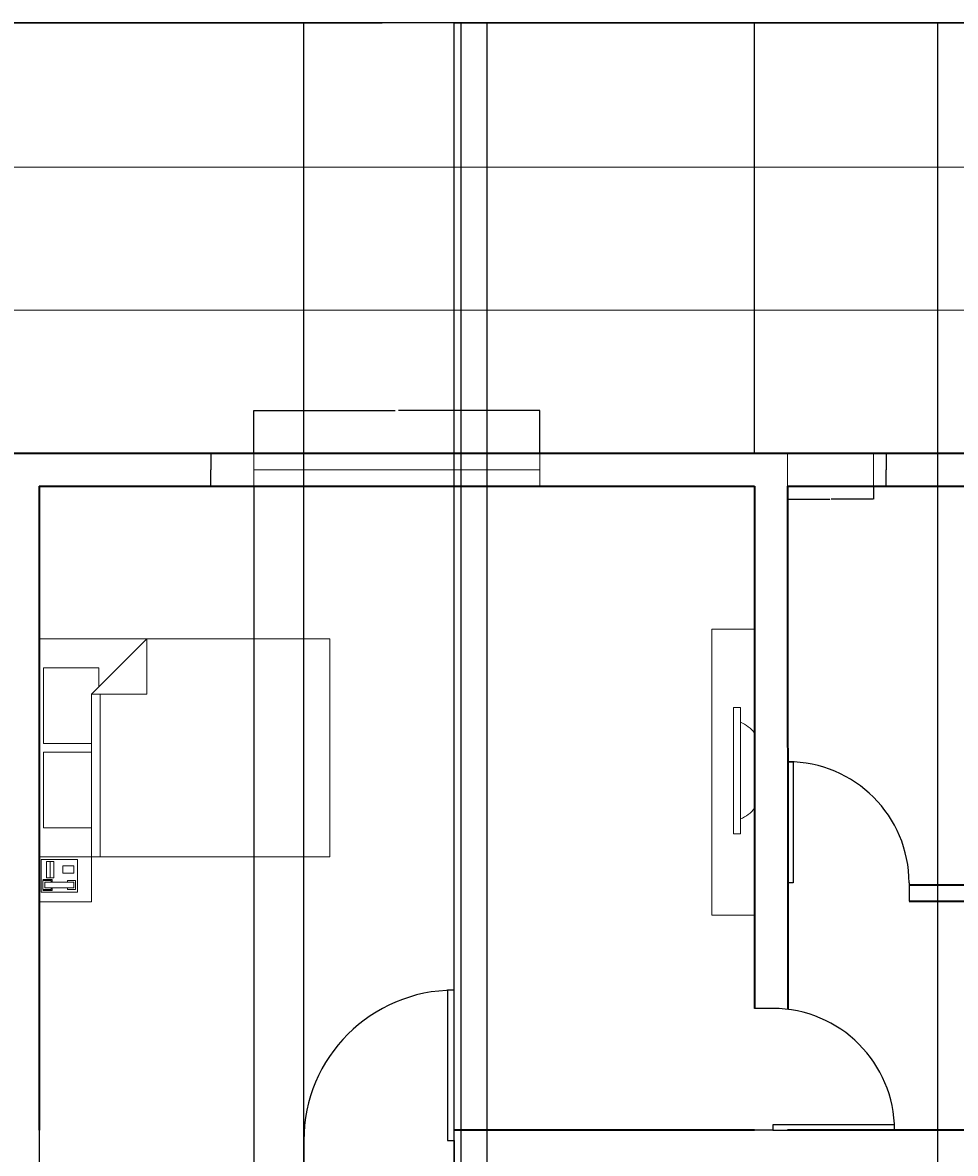
# Model space of a CAD drawing. Units: millimetres. Extents: x -8052 to 19968, y -37825 to -17505.
# Tile 8 of 10: x 4015 to 10533, y -25407 to -17505. Entities that reach past the tile are written whole.
import ezdxf

# ---------------------------------------------------------------- set-up
doc = ezdxf.new("R2010")
doc.units = ezdxf.units.MM
doc.header["$MEASUREMENT"] = 0
for name, color, linetype, lineweight in [('A-ANNO-DIMS', 2, 'Continuous', 18), ('A-DOOR', 3, 'Continuous', 25), ('A-EQPM', 8, 'Continuous', 18), ('A-FLOR', 8, 'Continuous', 18), ('A-FURN', 8, 'Continuous', 18), ('A-GLAZ', 4, 'Continuous', 18), ('A-WALL', 7, 'Continuous', 35)]:
    doc.layers.add(name, color=color, linetype=linetype, lineweight=lineweight)
doc.styles.get("Standard").update_dxf_attribs({"font": 'arial.ttf'})
doc.dimstyles.get("Standard").update_dxf_attribs({"dimtxt": 1.054, "dimasz": 1.055, "dimexe": 0.18, "dimexo": 0.0625, "dimgap": 0.09, "dimtad": 0, "dimtih": 1, "dimtoh": 1, "dimdec": 4, "dimzin": 0, "dimdsep": 46, "dimtxsty": 'Standard', "dimcen": 0.09, "dimadec": 0, "dimazin": 0, "dimtfac": 1, "dimtdec": 4, "dimtofl": 0, "dimtmove": 0, "dimatfit": 3, "dimfxl": 1, "dimtolj": 1, "dimtzin": 0, "dimarcsym": 0})

# ---------------------------------------------------------------- blocks, each defined once
blk = doc.blocks.new('*U9')
for p, q in [((-40, 0), (-40, 6)), ((0, 0), (0, 6))]:
    blk.add_line(p, q)
blk.add_lwpolyline([(0, 0), (0, -40), (-1.75, -40), (-1.75, 0)], close=True)
blk.add_arc((0, 0), 40, 180, 270)
blk = doc.blocks.new('Bed - Queen')
for p, q in [((0, -80.00003), (0, 0)), ((0, 0), (59.99999, 0)), ((59.99999, 0), (59.99999, -80.00003)), ((7.99999, -1.2), (28.79998, -1.2)), ((7.99999, -14.4), (7.99999, -1.2)), ((28.79998, -1.2), (28.79998, -14.4)), ((31.19999, -1.2), (51.99999, -1.2)), ((31.19999, -14.4), (31.19999, -1.2)), ((51.99999, -1.2), (51.99999, -16.4)), ((0, -14.4), (44.8, -14.4)), ((59.99999, -29.6), (44.8, -14.4)), ((44.8, -14.4), (44.8, -29.6)), ((44.8, -16.8), (0, -16.8)), ((51.99999, -16.4), (46.79936, -16.4)), ((44.8, -29.6), (59.99999, -29.6)), ((59.99999, -80.00003), (0, -80.00003))]:
    blk.add_line(p, q)
blk = doc.blocks.new('Phone - Desk')
for p, q in [((-4.5, -5), (-4.5, 5)), ((-4.5, 5), (4.5, 5)), ((-4, 4.5), (-4, 2)), ((-3.75, 4.5), (-3.75, 2.25)), ((-1.25, 4.5), (-3.75, 4.5)), ((-3.25, 4), (-3.25, -4)), ((-3.25, 4), (-1.75, 4)), ((-1.75, -4), (-1.75, 4)), ((-1.25, 2.25), (-1.25, 4.5)), ((-1, 2), (-1, 4.5)), ((4, 3.5), (-0.5, 3.5)), ((-0.5, 3.5), (-0.5, 1.5)), ((4, 1.5), (4, 3.5)), ((4.5, 5), (4.5, -5)), ((-4, 2), (-3.25, 2)), ((-3.75, 2.25), (-3.25, 2.25)), ((-1.75, 2.25), (-1.25, 2.25)), ((-1.75, 2), (-1, 2)), ((-0.5, 2.5), (4, 2.5)), ((-0.5, 1.5), (4, 1.5)), ((-3.75, -2.25), (-3.25, -2.25)), ((-3.75, -4.5), (-3.75, -2.25)), ((-1.75, -2.25), (-1.25, -2.25)), ((-1.25, -2.25), (-1.25, -4.5)), ((2.75, -1), (0.75, -1)), ((0.75, -1), (0.75, -4)), ((2.75, -4), (2.75, -1)), ((4.5, -5), (-4.5, -5)), ((-1.25, -4.5), (-3.75, -4.5)), ((-3.25, -4), (-1.75, -4)), ((0.75, -4), (2.75, -4))]:
    blk.add_line(p, q)
blk = doc.blocks.new('*U20')
for p, q in [((0, 0), (0, -6)), ((-40, 0), (-40, -6))]:
    blk.add_line(p, q)
blk.add_lwpolyline([(0, 0), (0, 40), (-1.75, 40), (-1.75, 0)], close=True)
blk.add_arc((0, 0), 40, 90, 180)
blk = doc.blocks.new('TABLE-BEDSIDE')
for p, q in [((365.8, 315.3), (365.8, 0)), ((365.8, 0), (0, 0))]:
    blk.add_line(p, q)
blk = doc.blocks.new('MEDIA-CONSOLE-2000')
for points in [[(300, 2000), (0, 2000), (0, 0), (300, 0)], [(201.6, 1452.1), (152.5, 1452.1), (152.5, 569.2), (201.6, 569.2)], [(201.6, 569.2), (152.5, 569.2), (152.5, 1452.1), (201.6, 1452.1)]]:
    blk.add_lwpolyline(points, close=True)
for centre, start, end in [((115.1, 1133.4), 37.07446, 68.10078), ((115.1, 887.8), 291.89922, 322.92554)]:
    blk.add_arc(centre, 231.7, start, end)
blk = doc.blocks.new('DOOR-SWING-850')
for p, q in [((0, 127.5), (0, 0)), ((850, 127.5), (850, 0))]:
    blk.add_line(p, q)
blk.add_lwpolyline([(850, 127.5), (850, 977.5), (812.8, 977.5), (812.8, 127.5)], close=True)
blk.add_arc((850, 127.5), 850, 90, 180)
blk = doc.blocks.new('WIN-2000')
for p, q in [((0, 0), (0, 230)), ((2000, 0), (2000, 230)), ((0, 115), (2000, 115))]:
    blk.add_line(p, q)
blk = doc.blocks.new('VENT-OPENING-600')
for p, q in [((0, 0), (0, 230)), ((600, 0), (600, 230))]:
    blk.add_line(p, q)
blk = doc.blocks.new('*D52')
at = {"layer": 'A-ANNO-DIMS', "color": 0, "lineweight": -2, "transparency": 16777216}
for p, q in [((5630, -20514.8), (5630, -20214.7)), ((5631, -20214.8), (6619.1, -20214.8)), ((7628.9, -20214.8), (6640.9, -20214.8)), ((7630, -20514.8), (7630, -20214.7))]:
    blk.add_line(p, q, dxfattribs=at)
at = {"layer": 'A-ANNO-DIMS', "color": 0, "lineweight": 100, "transparency": 16777216}
for points in [[(5631, -20214.7), (5631, -20215), (5630, -20214.8)], [(7628.9, -20214.7), (7628.9, -20215), (7630, -20214.8)]]:
    blk.add_solid(points, dxfattribs=at)
at = {"layer": 'Defpoints', "color": 0, "lineweight": 100, "transparency": 16777216}
for p in [(5630, -20214.8), (5630, -20514.8), (7630, -20514.8)]:
    blk.add_point(p, dxfattribs=at)
at = {"layer": 'A-ANNO-DIMS', "color": 0, "transparency": 16777216, "insert": (6630, -20214.8), "char_height": 1.054, "attachment_point": 5}
blk.add_mtext('\\A1;BEDROOM WINDOW 2000 TYP.', dxfattribs=at)
blk = doc.blocks.new('*D53')
at = {"layer": 'A-ANNO-DIMS', "color": 0, "lineweight": -2, "transparency": 16777216}
for p, q in [((5629.9, -20514.8), (5329.8, -20514.8)), ((5330, -20515.9), (5330, -20629.2)), ((5330, -20743.8), (5330, -20630.5)), ((5629.9, -20744.8), (5329.8, -20744.8))]:
    blk.add_line(p, q, dxfattribs=at)
at = {"layer": 'A-ANNO-DIMS', "color": 0, "lineweight": 100, "transparency": 16777216}
for points in [[(5329.8, -20515.9), (5330.2, -20515.9), (5330, -20514.8)], [(5329.8, -20743.8), (5330.2, -20743.8), (5330, -20744.8)]]:
    blk.add_solid(points, dxfattribs=at)
at = {"layer": 'Defpoints', "color": 0, "lineweight": 100, "transparency": 16777216}
for p in [(5630, -20514.8), (5330, -20744.8), (5630, -20744.8)]:
    blk.add_point(p, dxfattribs=at)
at = {"layer": 'A-ANNO-DIMS', "color": 0, "transparency": 16777216, "insert": (5330, -20629.8), "char_height": 1.054, "attachment_point": 5}
blk.add_mtext('\\A1;230 TYP.', dxfattribs=at)
blk = doc.blocks.new('*D64')
at = {"layer": 'A-ANNO-DIMS', "color": 0, "lineweight": -2, "transparency": 16777216}
for p, q in [((9360, -20744.9), (9360, -20835)), ((9960, -20744.9), (9960, -20835)), ((9361, -20834.8), (9654.7, -20834.8)), ((9958.9, -20834.8), (9665.2, -20834.8))]:
    blk.add_line(p, q, dxfattribs=at)
at = {"layer": 'A-ANNO-DIMS', "color": 0, "lineweight": 100, "transparency": 16777216}
for points in [[(9361, -20834.7), (9361, -20835), (9360, -20834.8)], [(9958.9, -20834.7), (9958.9, -20835), (9960, -20834.8)]]:
    blk.add_solid(points, dxfattribs=at)
at = {"layer": 'Defpoints', "color": 0, "lineweight": 100, "transparency": 16777216}
for p in [(9360, -20744.8), (9960, -20744.8), (9960, -20834.8)]:
    blk.add_point(p, dxfattribs=at)
at = {"layer": 'A-ANNO-DIMS', "color": 0, "transparency": 16777216, "insert": (9660, -20834.8), "char_height": 1.054, "attachment_point": 5}
blk.add_mtext('\\A1;VENT 600 TYP.', dxfattribs=at)
blk = doc.blocks.new('*D65')
at = {"layer": 'A-ANNO-DIMS', "color": 0, "lineweight": -2, "transparency": 16777216}
for p, q in [((9960, -20514.8), (10050.2, -20514.8)), ((10050, -20515.9), (10050, -20629.2)), ((10050, -20743.8), (10050, -20630.5)), ((9960, -20744.8), (10050.2, -20744.8))]:
    blk.add_line(p, q, dxfattribs=at)
at = {"layer": 'A-ANNO-DIMS', "color": 0, "lineweight": 100, "transparency": 16777216}
for points in [[(10049.8, -20515.9), (10050.2, -20515.9), (10050, -20514.8)], [(10049.8, -20743.8), (10050.2, -20743.8), (10050, -20744.8)]]:
    blk.add_solid(points, dxfattribs=at)
at = {"layer": 'Defpoints', "color": 0, "lineweight": 100, "transparency": 16777216}
for p in [(9960, -20514.8), (10050, -20514.8), (9960, -20744.8)]:
    blk.add_point(p, dxfattribs=at)
at = {"layer": 'A-ANNO-DIMS', "color": 0, "transparency": 16777216, "insert": (10050, -20629.8), "char_height": 1.054, "attachment_point": 5}
blk.add_mtext('\\A1;230 TYP.', dxfattribs=at)
blk = doc.blocks.new('*D84')
at = {"layer": 'A-ANNO-DIMS', "color": 0, "lineweight": -2, "transparency": 16777216}
for p, q in [((-7040, -18514.8), (-7040, -17505.2)), ((-7039, -17505.3), (3022.9, -17505.3)), ((13088.9, -17505.3), (3027.1, -17505.3)), ((13090, -18514.8), (13090, -17505.2))]:
    blk.add_line(p, q, dxfattribs=at)
at = {"layer": 'A-ANNO-DIMS', "color": 0, "lineweight": 100, "transparency": 16777216}
for points in [[(-7039, -17505.2), (-7039, -17505.5), (-7040, -17505.3)], [(13088.9, -17505.2), (13088.9, -17505.5), (13090, -17505.3)]]:
    blk.add_solid(points, dxfattribs=at)
at = {"layer": 'Defpoints', "color": 0, "lineweight": 100, "transparency": 16777216}
for p in [(13090, -17505.3), (-7040, -18514.8), (13090, -18514.8)]:
    blk.add_point(p, dxfattribs=at)
at = {"layer": 'A-ANNO-DIMS', "color": 0, "transparency": 16777216, "insert": (3025, -17505.3), "char_height": 1.05, "attachment_point": 5}
blk.add_mtext('\\A1;20130', dxfattribs=at)
blk = doc.blocks.new('*D92')
at = {"layer": 'A-ANNO-DIMS', "color": 0, "lineweight": -2, "transparency": 16777216}
for p, q in [((3900, -20514.8), (3900, -17505.2)), ((3901, -17505.3), (6513.3, -17505.3)), ((9128.9, -17505.3), (6516.6, -17505.3)), ((9130, -20514.8), (9130, -17505.2))]:
    blk.add_line(p, q, dxfattribs=at)
at = {"layer": 'A-ANNO-DIMS', "color": 0, "lineweight": 100, "transparency": 16777216}
for points in [[(3901, -17505.2), (3901, -17505.5), (3900, -17505.3)], [(9128.9, -17505.2), (9128.9, -17505.5), (9130, -17505.3)]]:
    blk.add_solid(points, dxfattribs=at)
at = {"layer": 'Defpoints', "color": 0, "lineweight": 100, "transparency": 16777216}
for p in [(9130, -17505.3), (3900, -20514.8), (9130, -20514.8)]:
    blk.add_point(p, dxfattribs=at)
at = {"layer": 'A-ANNO-DIMS', "color": 0, "transparency": 16777216, "insert": (6515, -17505.3), "char_height": 1.05, "attachment_point": 5}
blk.add_mtext('\\A1;5230', dxfattribs=at)
blk = doc.blocks.new('*D93')
at = {"layer": 'A-ANNO-DIMS', "color": 0, "lineweight": -2, "transparency": 16777216}
for p, q in [((9130, -20514.8), (9130, -17505.2)), ((9131, -17505.3), (10608.3, -17505.3)), ((12088.9, -17505.3), (10611.7, -17505.3)), ((12090, -20514.8), (12090, -17505.2))]:
    blk.add_line(p, q, dxfattribs=at)
at = {"layer": 'A-ANNO-DIMS', "color": 0, "lineweight": 100, "transparency": 16777216}
for points in [[(9131, -17505.2), (9131, -17505.5), (9130, -17505.3)], [(12088.9, -17505.2), (12088.9, -17505.5), (12090, -17505.3)]]:
    blk.add_solid(points, dxfattribs=at)
at = {"layer": 'Defpoints', "color": 0, "lineweight": 100, "transparency": 16777216}
for p in [(12090, -17505.3), (9130, -20514.8), (12090, -20514.8)]:
    blk.add_point(p, dxfattribs=at)
at = {"layer": 'A-ANNO-DIMS', "color": 0, "transparency": 16777216, "insert": (10610, -17505.3), "char_height": 1.05, "attachment_point": 5}
blk.add_mtext('\\A1;2960', dxfattribs=at)
blk = doc.blocks.new('*D95')
at = {"layer": 'A-ANNO-DIMS', "color": 0, "lineweight": -2, "transparency": 16777216}
for p, q in [((4130, -20744.9), (4130, -37824.5)), ((5630, -20744.9), (5630, -37824.5)), ((4131, -37824.3), (4878.4, -37824.3)), ((5628.9, -37824.3), (4881.6, -37824.3))]:
    blk.add_line(p, q, dxfattribs=at)
at = {"layer": 'A-ANNO-DIMS', "color": 0, "lineweight": 100, "transparency": 16777216}
for points in [[(4131, -37824.2), (4131, -37824.5), (4130, -37824.3)], [(5628.9, -37824.2), (5628.9, -37824.5), (5630, -37824.3)]]:
    blk.add_solid(points, dxfattribs=at)
at = {"layer": 'Defpoints', "color": 0, "lineweight": 100, "transparency": 16777216}
for p in [(4130, -20744.8), (5630, -20744.8), (5630, -37824.3)]:
    blk.add_point(p, dxfattribs=at)
at = {"layer": 'A-ANNO-DIMS', "color": 0, "transparency": 16777216, "insert": (4880, -37824.3), "char_height": 1.05, "attachment_point": 5}
blk.add_mtext('\\A1;1500', dxfattribs=at)
blk = doc.blocks.new('*D104')
at = {"layer": 'A-ANNO-DIMS', "color": 0, "lineweight": -2, "transparency": 16777216}
for p, q in [((5980, -35400), (5980, -17505.2)), ((5981, -17505.3), (6528.4, -17505.3)), ((7078.9, -17505.3), (6531.6, -17505.3)), ((7080, -35584.8), (7080, -17505.2))]:
    blk.add_line(p, q, dxfattribs=at)
at = {"layer": 'A-ANNO-DIMS', "color": 0, "lineweight": 100, "transparency": 16777216}
for points in [[(5981, -17505.2), (5981, -17505.5), (5980, -17505.3)], [(7078.9, -17505.2), (7078.9, -17505.5), (7080, -17505.3)]]:
    blk.add_solid(points, dxfattribs=at)
at = {"layer": 'Defpoints', "color": 0, "lineweight": 100, "transparency": 16777216}
for p in [(7080, -17505.3), (5980, -35400), (7080, -35584.8)]:
    blk.add_point(p, dxfattribs=at)
at = {"layer": 'A-ANNO-DIMS', "color": 0, "transparency": 16777216, "insert": (6530, -17505.3), "char_height": 1.05, "attachment_point": 5}
blk.add_mtext('\\A1;1100', dxfattribs=at)
blk = doc.blocks.new('*D108')
at = {"layer": 'A-ANNO-DIMS', "color": 0, "lineweight": -2, "transparency": 16777216}
for p, q in [((-330, -29974.8), (-330, -17505.2)), ((-329, -17505.3), (3348.3, -17505.3)), ((7028.9, -17505.3), (3351.6, -17505.3)), ((7030, -29974.8), (7030, -17505.2))]:
    blk.add_line(p, q, dxfattribs=at)
at = {"layer": 'A-ANNO-DIMS', "color": 0, "lineweight": 100, "transparency": 16777216}
for points in [[(-329, -17505.2), (-329, -17505.5), (-330, -17505.3)], [(7028.9, -17505.2), (7028.9, -17505.5), (7030, -17505.3)]]:
    blk.add_solid(points, dxfattribs=at)
at = {"layer": 'Defpoints', "color": 0, "lineweight": 100, "transparency": 16777216}
for p in [(7030, -17505.3), (-330, -29974.8), (7030, -29974.8)]:
    blk.add_point(p, dxfattribs=at)
at = {"layer": 'A-ANNO-DIMS', "color": 0, "transparency": 16777216, "insert": (3350, -17505.3), "char_height": 1.05, "attachment_point": 5}
blk.add_mtext('\\A1;7360', dxfattribs=at)
blk = doc.blocks.new('*D123')
at = {"layer": 'A-ANNO-DIMS', "color": 0, "lineweight": -2, "transparency": 16777216}
for p, q in [((7260, -25474.8), (7260, -17505.2)), ((7261, -17505.3), (9673.3, -17505.3)), ((12088.9, -17505.3), (9676.7, -17505.3)), ((12090, -25474.8), (12090, -17505.2))]:
    blk.add_line(p, q, dxfattribs=at)
at = {"layer": 'A-ANNO-DIMS', "color": 0, "lineweight": 100, "transparency": 16777216}
for points in [[(7261, -17505.2), (7261, -17505.5), (7260, -17505.3)], [(12088.9, -17505.2), (12088.9, -17505.5), (12090, -17505.3)]]:
    blk.add_solid(points, dxfattribs=at)
at = {"layer": 'Defpoints', "color": 0, "lineweight": 100, "transparency": 16777216}
for p in [(7260, -17505.3), (7260, -25474.8), (12090, -25474.8)]:
    blk.add_point(p, dxfattribs=at)
at = {"layer": 'A-ANNO-DIMS', "color": 0, "transparency": 16777216, "insert": (9675, -17505.3), "char_height": 1.05, "attachment_point": 5}
blk.add_mtext('\\A1;4830', dxfattribs=at)
blk = doc.blocks.new('*D124')
at = {"layer": 'A-ANNO-DIMS', "color": 0, "lineweight": -2, "transparency": 16777216}
for p, q in [((7030, -29974.8), (7030, -17505.2)), ((7031, -17505.3), (8718.3, -17505.3)), ((10408.9, -17505.3), (8721.6, -17505.3)), ((10410, -29974.8), (10410, -17505.2))]:
    blk.add_line(p, q, dxfattribs=at)
at = {"layer": 'A-ANNO-DIMS', "color": 0, "lineweight": 100, "transparency": 16777216}
for points in [[(7031, -17505.2), (7031, -17505.5), (7030, -17505.3)], [(10408.9, -17505.2), (10408.9, -17505.5), (10410, -17505.3)]]:
    blk.add_solid(points, dxfattribs=at)
at = {"layer": 'Defpoints', "color": 0, "lineweight": 100, "transparency": 16777216}
for p in [(10410, -17505.3), (7030, -29974.8), (10410, -29974.8)]:
    blk.add_point(p, dxfattribs=at)
at = {"layer": 'A-ANNO-DIMS', "color": 0, "transparency": 16777216, "insert": (8720, -17505.3), "char_height": 1.05, "attachment_point": 5}
blk.add_mtext('\\A1;3380', dxfattribs=at)

msp = doc.modelspace()

# ---------------------------------------------------------------- linework, layer by layer
at = {"layer": 'A-DOOR'}
msp.add_line((9359.979, -23517.343), (9359.979, -23644.843), dxfattribs=at)
at = {"layer": 'A-FLOR'}
for p, q in [((-4810.021, -18514.843), (13089.979, -18514.843)), ((-6040.021, -19514.843), (12089.979, -19514.843))]:
    msp.add_line(p, q, dxfattribs=at)
at = {"layer": 'A-WALL'}
for p, q in [((3899.979, -20514.843), (4129.979, -20514.843)), ((4129.979, -20514.843), (9129.979, -20514.843)), ((9129.979, -20514.843), (9359.979, -20514.843)), ((9359.979, -20514.843), (11859.979, -20514.843)), ((4129.979, -20744.843), (9129.979, -20744.843)), ((4129.979, -20744.843), (4129.979, -25244.843)), ((9129.979, -20744.843), (9129.979, -24394.843)), ((9359.979, -20744.843), (11859.979, -20744.843)), ((9359.979, -20744.843), (9361.771, -24401.265)), ((9359.979, -23529.843), (9361.401, -23529.843)), ((10209.02, -23529.843), (11859.979, -23529.843)), ((9359.979, -23644.843), (9361.401, -23644.843)), ((10209.02, -23644.843), (11859.979, -23644.843)), ((9129.979, -25244.843), (7029.979, -25244.843)), ((11859.979, -25244.843), (9359.979, -25244.843))]:
    msp.add_line(p, q, dxfattribs=at)

# ---------------------------------------------------------------- block references
at = {"layer": 'A-DOOR', "xscale": 21.1904853351297, "yscale": 21.1904853351297, "zscale": 21.1904853351297, "rotation": 180}
msp.add_blockref('*U9', (9361.401, -23517.7), dxfattribs=at)
at = {"layer": 'A-DOOR', "xscale": 26.25, "yscale": 26.25, "zscale": 26.25}
msp.add_blockref('*U20', (7029.979, -25317.343), dxfattribs=at)
at = {"layer": 'A-DOOR', "rotation": 270.0000000000442}
msp.add_blockref('DOOR-SWING-850', (9129.979, -24394.843), dxfattribs=at)
at = {"layer": 'A-EQPM'}
msp.add_blockref('MEDIA-CONSOLE-2000', (8829.979, -23742.93), dxfattribs=at)
at = {"layer": 'A-EQPM', "xscale": 25.4, "yscale": 25.4, "zscale": 25.4, "rotation": 90}
msp.add_blockref('Phone - Desk', (4271.24, -23468.572), dxfattribs=at)
at = {"layer": 'A-FURN', "xscale": 25.4, "yscale": 25.4, "zscale": 25.4, "rotation": 90}
msp.add_blockref('Bed - Queen', (4129.979, -23334.944), dxfattribs=at)
at = {"layer": 'A-FURN'}
msp.add_blockref('TABLE-BEDSIDE', (4129.979, -23650.203), dxfattribs=at)
at = {"layer": 'A-GLAZ', "rotation": 180}
msp.add_blockref('WIN-2000', (7629.98, -20514.843), dxfattribs=at)
at = {"layer": 'A-GLAZ'}
msp.add_blockref('VENT-OPENING-600', (9359.979, -20744.843), dxfattribs=at)

# ---------------------------------------------------------------- dimensions: what is measured, and where the dimension line sits
at = {"layer": 'A-ANNO-DIMS'}
for base, p1, p2, picture, middle in [((13089.979, -17505.343), (-7040.021, -18514.843), (13089.979, -18514.843), '*D84', (3024.979, -17505.343)), ((7029.979, -17505.343), (-330.021, -29974.843), (7029.979, -29974.843), '*D108', (3349.979, -17505.343)), ((9129.979, -17505.343), (3899.979, -20514.843), (9129.979, -20514.843), '*D92', (6514.979, -17505.343)), ((7079.979, -17505.343), (5979.979, -35400.039), (7079.979, -35584.843), '*D104', (6529.979, -17505.343)), ((10409.979, -17505.343), (7029.979, -29974.843), (10409.979, -29974.843), '*D124', (8719.979, -17505.343)), ((7259.979, -17505.343), (12089.979, -25474.843), (7259.979, -25474.843), '*D123', (9674.979, -17505.343)), ((12089.979, -17505.343), (9129.979, -20514.843), (12089.979, -20514.843), '*D93', (10609.979, -17505.343)), ((5629.979, -37824.343), (4129.979, -20744.843), (5629.979, -20744.843), '*D95', (4879.979, -37824.343))]:
    dim = msp.add_linear_dim(base=base, p1=p1, p2=p2, dimstyle='Standard', override={"dimdec": 0, "dimlfac": 1, "dimrnd": 0, "dimzin": 0, "dimdsep": 46, "dimlunit": 2}, dxfattribs=at)
    dim.commit()
    dim.dimension.update_dxf_attribs({"geometry": picture, "text_midpoint": middle})
for base, p1, p2, angle, text, picture, middle in [((5629.979, -20214.843), (7629.979, -20514.843), (5629.979, -20514.843), 180, 'BEDROOM WINDOW <> TYP.', '*D52', (6629.979, -20214.843)), ((5329.979, -20744.843), (5629.979, -20514.843), (5629.979, -20744.843), 270, '<> TYP.', '*D53', (5329.979, -20629.843)), ((10049.979, -20514.843), (9959.979, -20744.843), (9959.979, -20514.843), 90, '<> TYP.', '*D65', (10049.979, -20629.843))]:
    dim = msp.add_linear_dim(base=base, p1=p1, p2=p2, angle=angle, text=text, dimstyle='Standard', override={"dimdec": 0, "dimlfac": 1, "dimrnd": 0, "dimzin": 0, "dimdsep": 46, "dimlunit": 2}, dxfattribs=at)
    dim.commit()
    dim.dimension.update_dxf_attribs({"geometry": picture, "text_midpoint": middle})
dim = msp.add_linear_dim(base=(9959.979, -20834.843), p1=(9359.979, -20744.843), p2=(9959.979, -20744.843), text='VENT <> TYP.', dimstyle='Standard', override={"dimdec": 0, "dimlfac": 1, "dimrnd": 0, "dimzin": 0, "dimdsep": 46, "dimlunit": 2}, dxfattribs=at)
dim.commit()
dim.dimension.update_dxf_attribs({"geometry": '*D64', "text_midpoint": (9659.979, -20834.843)})

doc.saveas('drawing.dxf')
